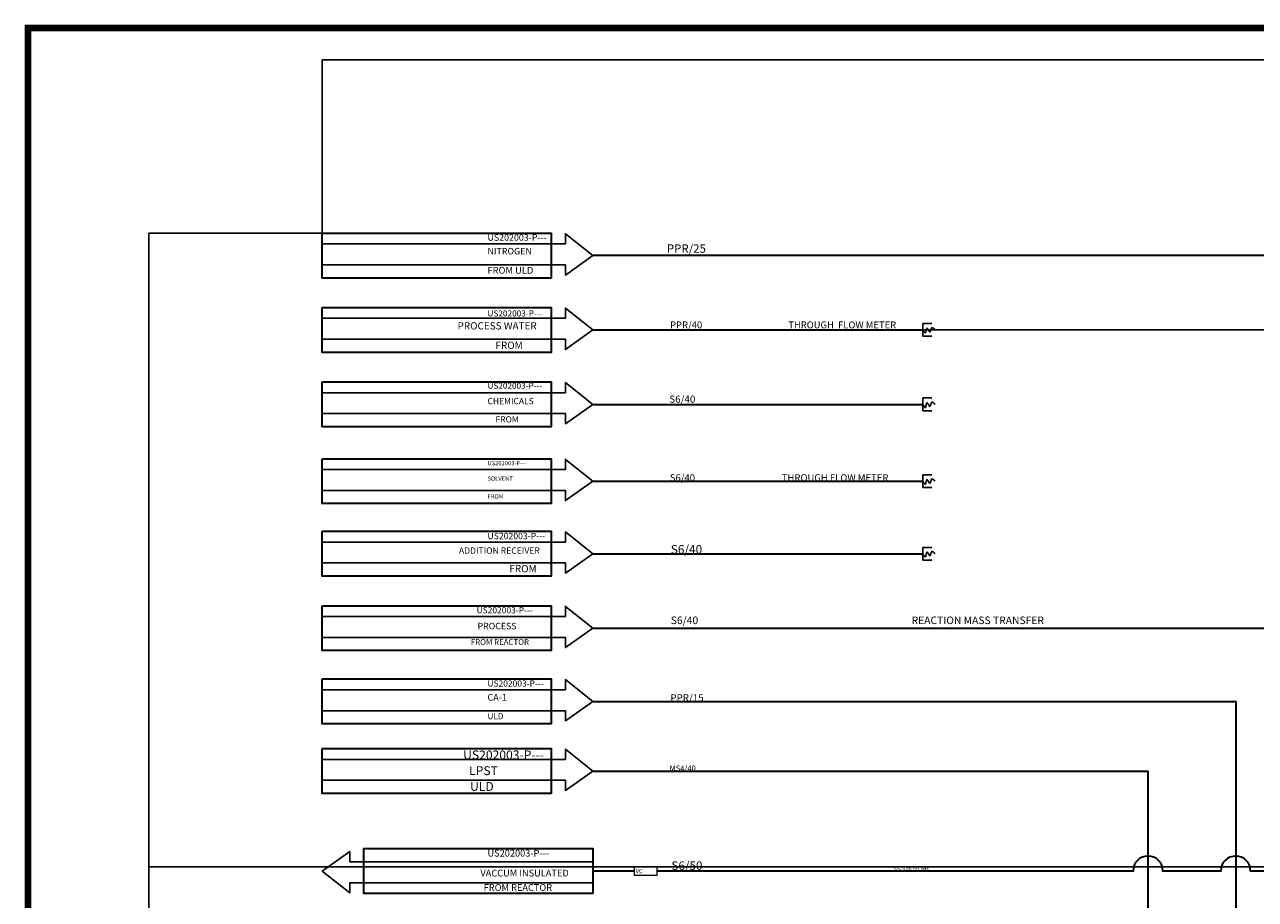
# Model space of a CAD drawing. Units: millimetres. Extents: x 353872 to 441597, y 126154 to 187356.
# Tile 18 of 28: x 353872 to 382257, y 167178 to 187356. Entities that reach past the tile are written whole.
import ezdxf

# ---------------------------------------------------------------- set-up
doc = ezdxf.new("R2010")
doc.units = ezdxf.units.MM
for name, color, linetype, lineweight in [('A-ANNO-DIMS', 2, 'Continuous', 18), ('P-ANNO-TEXT', 7, 'Continuous', 25), ('P-ANNO-TTLB', 7, 'Continuous', 25), ('P-EQPM', 5, 'Continuous', 35), ('P-INST-SIGN', 4, 'Continuous', 18), ('P-PIPE', 3, 'Continuous', 35), ('P-VALV', 2, 'Continuous', 25)]:
    doc.layers.add(name, color=color, linetype=linetype, lineweight=lineweight)
doc.styles.get("Standard").update_dxf_attribs({"font": 'arial.ttf'})
doc.dimstyles.get("Standard").update_dxf_attribs({"dimtxt": 0.18, "dimasz": 0.18, "dimexe": 0.18, "dimexo": 0.0625, "dimgap": 0.09, "dimtad": 0, "dimtih": 1, "dimtoh": 1, "dimdec": 4, "dimzin": 0, "dimdsep": 46, "dimtxsty": 'Standard', "dimcen": 0.09, "dimadec": 0, "dimazin": 0, "dimtfac": 1, "dimtdec": 4, "dimtofl": 0, "dimtmove": 0, "dimatfit": 3, "dimfxl": 1, "dimtolj": 1, "dimtzin": 0, "dimarcsym": 0})

# ---------------------------------------------------------------- blocks, each defined once
blk = doc.blocks.new('*D24')
at = {"layer": 'A-ANNO-DIMS', "color": 0, "lineweight": -2, "transparency": 16777216}
for p, q in [((360737, 182546), (360737, 186546)), ((360737, 186546), (396698, 186546)), ((432661, 186546), (396699, 186546)), ((432661, 177114), (432661, 186546))]:
    blk.add_line(p, q, dxfattribs=at)
at = {"layer": 'A-ANNO-DIMS', "color": 0, "transparency": 16777216}
for points in [[(360737, 186546), (360737, 186546), (360737, 186546)], [(432661, 186546), (432661, 186546), (432661, 186546)]]:
    blk.add_solid(points, dxfattribs=at)
at = {"layer": 'Defpoints', "color": 0, "transparency": 16777216}
for p in [(432661, 186546), (360737, 182546), (432661, 177114)]:
    blk.add_point(p, dxfattribs=at)
at = {"layer": 'A-ANNO-DIMS', "color": 0, "transparency": 16777216, "insert": (396699, 186546), "char_height": 0.18, "attachment_point": 5}
blk.add_mtext('\\A1;71924', dxfattribs=at)
blk = doc.blocks.new('*D25')
at = {"layer": 'A-ANNO-DIMS', "color": 0, "lineweight": -2, "transparency": 16777216}
for p, q in [((360736, 182546), (356736, 182546)), ((356737, 182546), (356737, 160180)), ((356737, 137813), (356737, 160179)), ((361696, 137813), (356736, 137813))]:
    blk.add_line(p, q, dxfattribs=at)
at = {"layer": 'A-ANNO-DIMS', "color": 0, "transparency": 16777216}
for points in [[(356737, 182546), (356737, 182546), (356737, 182546)], [(356737, 137813), (356737, 137813), (356737, 137813)]]:
    blk.add_solid(points, dxfattribs=at)
at = {"layer": 'Defpoints', "color": 0, "transparency": 16777216}
for p in [(360737, 182546), (356737, 137813), (361696, 137813)]:
    blk.add_point(p, dxfattribs=at)
at = {"layer": 'A-ANNO-DIMS', "color": 0, "transparency": 16777216, "insert": (356737, 160179), "char_height": 0.18, "attachment_point": 5}
blk.add_mtext('\\A1;44733', dxfattribs=at)
blk = doc.blocks.new('*D28')
at = {"layer": 'A-ANNO-DIMS', "color": 0, "lineweight": -2, "transparency": 16777216}
for p, q in [((366977, 182028), (440591, 182028)), ((440591, 182028), (440591, 181171)), ((440591, 180314), (440591, 181171)), ((366977, 180314), (440591, 180314))]:
    blk.add_line(p, q, dxfattribs=at)
at = {"layer": 'A-ANNO-DIMS', "color": 0, "transparency": 16777216}
for points in [[(440591, 182028), (440591, 182028), (440591, 182028)], [(440591, 180314), (440591, 180314), (440591, 180314)]]:
    blk.add_solid(points, dxfattribs=at)
at = {"layer": 'Defpoints', "color": 0, "transparency": 16777216}
for p in [(366977, 182028), (366977, 180314), (440591, 180314)]:
    blk.add_point(p, dxfattribs=at)
at = {"layer": 'A-ANNO-DIMS', "color": 0, "transparency": 16777216, "insert": (440591, 181171), "char_height": 0.18, "attachment_point": 5}
blk.add_mtext('\\A1;1714.5', dxfattribs=at)
blk = doc.blocks.new('*D34')
at = {"layer": 'A-ANNO-DIMS', "color": 0, "lineweight": -2, "transparency": 16777216}
for p, q in [((399457, 167930), (356736, 167930)), ((356737, 167930), (356737, 163994)), ((356737, 160058), (356737, 163994)), ((399457, 160058), (356736, 160058))]:
    blk.add_line(p, q, dxfattribs=at)
at = {"layer": 'A-ANNO-DIMS', "color": 0, "transparency": 16777216}
for points in [[(356737, 167930), (356737, 167930), (356737, 167930)], [(356737, 160058), (356737, 160058), (356737, 160058)]]:
    blk.add_solid(points, dxfattribs=at)
at = {"layer": 'Defpoints', "color": 0, "transparency": 16777216}
for p in [(399457, 167930), (356737, 160058), (399457, 160058)]:
    blk.add_point(p, dxfattribs=at)
at = {"layer": 'A-ANNO-DIMS', "color": 0, "transparency": 16777216, "insert": (356737, 163994), "char_height": 0.18, "attachment_point": 5}
blk.add_mtext('\\A1;7872', dxfattribs=at)

msp = doc.modelspace()

# ---------------------------------------------------------------- linework, layer by layer
at = {"layer": 'P-ANNO-TTLB', "const_width": 152.43}
msp.add_lwpolyline([(353948.03, 187280.05), (353948.03, 126916.34), (440835.19, 126916.34), (440835.19, 187280.05)], close=True, dxfattribs=at)
at = {"layer": 'P-ANNO-TTLB'}
for points in [[(360736.55, 181814.35), (366343.35, 181814.35), (366343.35, 181580.37), (366976.76, 182028.44), (366343.35, 182531.49), (366343.35, 182297.51), (360736.55, 182297.51)], [(360736.55, 180099.82), (366343.35, 180099.82), (366343.35, 179865.84), (366976.76, 180313.91), (366343.35, 180816.96), (366343.35, 180582.98), (360736.55, 180582.98)], [(360736.55, 178382.68), (366343.35, 178382.68), (366343.35, 178148.7), (366976.76, 178596.77), (366343.35, 179099.81), (366343.35, 178865.83), (360736.55, 178865.83)], [(360736.55, 176610.14), (366343.35, 176610.14), (366343.35, 176376.16), (366976.76, 176824.23), (366343.35, 177327.27), (366343.35, 177093.29), (360736.55, 177093.29)], [(360736.55, 174937.4), (366343.35, 174937.4), (366343.35, 174703.42), (366976.76, 175151.49), (366343.35, 175654.53), (366343.35, 175420.55), (360736.55, 175420.55)], [(360736.55, 173220.25), (366343.35, 173220.25), (366343.35, 172986.27), (366976.76, 173434.34), (366343.35, 173937.38), (366343.35, 173703.4), (360736.55, 173703.4)], [(360736.55, 171530.8), (366343.35, 171530.8), (366343.35, 171296.82), (366976.76, 171744.89), (366343.35, 172247.93), (366343.35, 172013.95), (360736.55, 172013.95)], [(360736.55, 169924.44), (366343.35, 169924.44), (366343.35, 169690.46), (366976.76, 170138.53), (366343.35, 170641.57), (366343.35, 170407.59), (360736.55, 170407.59)], [(366976.76, 168046.69), (361369.95, 168046.69), (361369.95, 168280.67), (360736.55, 167832.6), (361369.95, 167329.55), (361369.95, 167563.53), (366976.76, 167563.53)]]:
    msp.add_lwpolyline(points, dxfattribs=at)
at = {"layer": 'P-EQPM'}
for points in [[(360736.55, 182546.05), (366017.52, 182546.05), (366017.52, 181510.83), (360736.55, 181510.83)], [(360736.55, 180831.53), (366017.52, 180831.53), (366017.52, 179796.3), (360736.55, 179796.3)], [(360736.55, 179114.38), (366017.52, 179114.38), (366017.52, 178079.16), (360736.55, 178079.16)], [(360736.55, 177341.84), (366017.52, 177341.84), (366017.52, 176306.62), (360736.55, 176306.62)], [(360736.55, 175669.1), (366017.52, 175669.1), (366017.52, 174633.87), (360736.55, 174633.87)], [(360736.55, 173951.95), (366017.52, 173951.95), (366017.52, 172916.73), (360736.55, 172916.73)], [(360736.55, 172262.5), (366017.52, 172262.5), (366017.52, 171227.28), (360736.55, 171227.28)], [(360736.55, 170656.14), (366017.52, 170656.14), (366017.52, 169620.91), (360736.55, 169620.91)], [(366976.76, 167314.99), (361695.78, 167314.99), (361695.78, 168350.21), (366976.76, 168350.21)]]:
    msp.add_lwpolyline(points, close=True, dxfattribs=at)
at = {"layer": 'P-INST-SIGN'}
msp.add_lwpolyline([(367938.03, 167937.08), (368453.37, 167937.08), (368453.37, 167728.12), (367938.03, 167728.12)], close=True, dxfattribs=at)
at = {"layer": 'P-PIPE'}
for p, q in [((366976.76, 180313.91), (374589.81, 180313.91)), ((366976.76, 178596.77), (374589.81, 178596.77)), ((366976.76, 176824.23), (374589.81, 176824.23)), ((366976.76, 175151.49), (374589.81, 175151.49))]:
    msp.add_line(p, q, dxfattribs=at)
for points in [[(391060.3, 150079.91), (391060.3, 182028.44), (390103.2, 182028.44), (366976.76, 182028.44)], [(366976.76, 173434.34), (386613.67, 173434.34), (388181.19, 173434.34), (388181.19, 163303.71)], [(366976.76, 171744.89), (381803.29, 171744.89), (381803.29, 150820.94), (381803.29, 147742.48), (377889.79, 147742.48)], [(366976.76, 170138.53), (379780.51, 170138.53), (379780.51, 150820.94)], [(367938.03, 167832.6), (366976.76, 167832.6)]]:
    msp.add_lwpolyline(points, dxfattribs=at)
msp.add_lwpolyline([(388213.21, 147045.52), (383375.2, 147045.17), (383375.2, 147045.17), (383375.2, 149602.24), (383375.2, 167832.6), (382147.59, 167832.6, 1), (381458.98, 167832.6), (380124.81, 167832.6, 1), (379436.2, 167832.6), (368453.37, 167832.6)], format="xyb", dxfattribs=at)
at = {"layer": 'P-VALV'}
for points in [[(374795.09, 180460.92), (374589.81, 180460.92), (374589.81, 180166.91), (374795.09, 180166.91)], [(374795.09, 178743.77), (374589.81, 178743.77), (374589.81, 178449.76), (374795.09, 178449.76)], [(374795.09, 176971.23), (374589.81, 176971.23), (374589.81, 176677.22), (374795.09, 176677.22)], [(374795.09, 175298.49), (374589.81, 175298.49), (374589.81, 175004.48), (374795.09, 175004.48)]]:
    msp.add_lwpolyline(points, dxfattribs=at)
for points in [[(374589.81, 180313.91), (374612.53, 180272.99), (374664.3, 180179.73), (374669.17, 180449.62), (374759.38, 180173.93), (374779.71, 180418.89), (374840.84, 180345.25), (374867.67, 180312.93)], [(374589.81, 178596.77), (374612.53, 178555.84), (374664.3, 178462.59), (374669.17, 178732.48), (374759.38, 178456.78), (374779.71, 178701.74), (374840.84, 178628.1), (374867.67, 178595.78)], [(374589.81, 176824.23), (374612.53, 176783.31), (374664.3, 176690.05), (374669.17, 176959.94), (374759.38, 176684.24), (374779.71, 176929.21), (374840.84, 176855.56), (374867.67, 176823.24)], [(374589.81, 175151.49), (374612.53, 175110.56), (374664.3, 175017.31), (374669.17, 175287.2), (374759.38, 175011.5), (374779.71, 175256.46), (374840.84, 175182.82), (374867.67, 175150.5)]]:
    msp.add_open_spline(points, degree=3, knots=[0, 0, 0, 0, 92.12866386, 209.95127675, 322.04103606, 435.13566174, 523.59598502, 523.59598502, 523.59598502, 523.59598502], dxfattribs=at)

# ---------------------------------------------------------------- texts
at = {"layer": 'P-ANNO-TEXT'}
for s, height, p in [('US202003-P---', 150.08, (364546.6, 182370.19)), ('PPR/25', 194.303, (368682.88, 182093.6)), ('NITROGEN', 150.323, (364546.6, 182054.87)), ('FROM ULD', 157.474, (364546.6, 181609.94)), ('US202003-P---', 139.5822, (364546.6, 180624.5)), ('PROCESS WATER', 168.1748, (363856.22, 180323.7)), ('PPR/40', 159.239, (368759.6, 180349.53)), ('THROUGH  FLOW METER', 159.2393, (371484.01, 180349.53)), ('FROM', 168.175, (364731.16, 179874.42)), ('US202003-P---', 139.1196, (364546.6, 178956.78)), ('CHEMICALS', 143.641, (364546.6, 178600.82)), ('S6/40', 165.919, (368740.61, 178632.97)), ('FROM', 143.641, (364731.76, 178179.69)), ('US202003-P---', 98.0901, (364546.6, 177192.26)), ('SOLVENT', 98.09, (364546.6, 176835.8)), ('S6/40', 160.479, (368752.55, 176824.23)), ('THROUGH FLOW METER', 160.4793, (371335.02, 176824.23)), ('FROM', 98.09, (364546.6, 176423.55)), ('US202003-P---', 146.3293, (364546.6, 175486.02)), ('ADDITION RECEIVER', 145.5384, (363887.82, 175151)), ('S6/40', 200.127, (368773.88, 175151.49)), ('FROM', 167.883, (365052.05, 174723.23)), ('US202003-P---', 142.6002, (364295.26, 173776.65)), ('PROCESS', 148.959, (364317.09, 173408.2)), ('S6/40', 174.561, (368773.88, 173528.05)), ('REACTION MASS TRANSFER', 174.561, (374327.35, 173528.05)), ('FROM REACTOR', 132.5602, (364164.15, 173048.99)), ('US202003-P---', 142.6994, (364546.6, 172086.01)), ('CA-1', 153.799, (364546.6, 171762.84)), ('PPR/15', 164.668, (368766.73, 171744.89)), ('ULD', 138.433, (364546.6, 171332.87)), ('US202003-P---', 204.9218, (363986.27, 170407.59)), ('LPST', 204.922, (364123.68, 170044.33)), ('MS4/40', 127.648, (368747.62, 170138.53)), ('ULD', 204.922, (364144.86, 169679.63)), ('US202003-P---', 155.9724, (364546.6, 168165.93)), ('S6/50', 197.571, (368789.71, 167858.26)), ('VACCUM INSULATED', 155.9724, (364383.53, 167706.05)), ('VC', 98.09, (367961.78, 167781.41)), ('S5-316 50 NB', 98.0901, (373906.58, 167832.6)), ('FROM REACTOR', 155.9724, (364459.87, 167373.8))]:
    msp.add_text(s, height=height, dxfattribs=at).set_placement(p)

# ---------------------------------------------------------------- dimensions: what is measured, and where the dimension line sits
at = {"layer": 'A-ANNO-DIMS'}
dim = msp.add_linear_dim(base=(432660.97, 186546.05), p1=(360736.55, 182546.05), p2=(432660.97, 177114.41), dimstyle='Standard', override={"dimdec": 0, "dimlfac": 1, "dimrnd": 0, "dimzin": 0, "dimdsep": 46, "dimlunit": 2}, dxfattribs=at)
dim.commit()
dim.dimension.update_dxf_attribs({"geometry": '*D24', "text_midpoint": (396698.76, 186546.05)})
for base, p1, p2, override, picture, middle in [((356736.55, 137812.84), (360736.55, 182546.05), (361695.78, 137812.84), {"dimdec": 0, "dimlfac": 1, "dimrnd": 0, "dimzin": 0, "dimdsep": 46, "dimlunit": 2}, '*D25', (356736.55, 160179.44)), ((440591, 180313.91), (366976.76, 182028.44), (366976.76, 180313.91), {"dimdec": 1, "dimlfac": 1, "dimrnd": 0, "dimzin": 0, "dimdsep": 46, "dimlunit": 2}, '*D28', (440591, 181171.18)), ((356736.55, 160058.19), (399457.15, 167929.97), (399457.15, 160058.19), {"dimdec": 0, "dimlfac": 1, "dimrnd": 0, "dimzin": 0, "dimdsep": 46, "dimlunit": 2}, '*D34', (356736.55, 163994.08))]:
    dim = msp.add_linear_dim(base=base, p1=p1, p2=p2, angle=90, dimstyle='Standard', override=override, dxfattribs=at)
    dim.commit()
    dim.dimension.update_dxf_attribs({"geometry": picture, "text_midpoint": middle})

doc.saveas('drawing.dxf')
